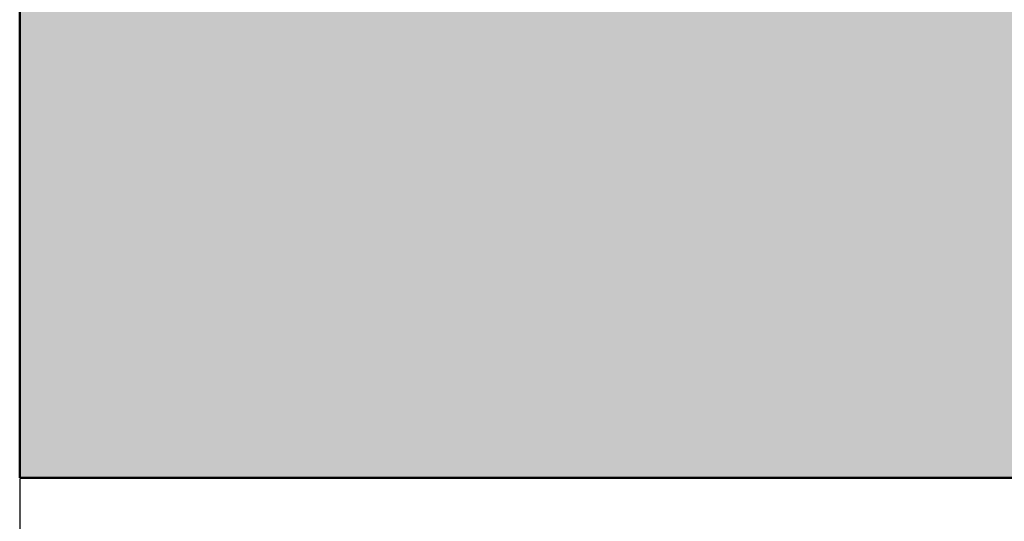
# Model space of a CAD drawing. Units: millimetres. Extents: x 0 to 2267, y 0 to 1823.
# Tile 12 of 256: x 1506 to 1590, y 1074 to 1116. Entities that reach past the tile are written whole.
import ezdxf

# ---------------------------------------------------------------- set-up
doc = ezdxf.new("R2010")
doc.units = ezdxf.units.MM
doc.header["$MEASUREMENT"] = 0
for name, color, linetype, lineweight in [('M-DIMS', 2, 'Continuous', 25), ('M-HATC', 252, 'Continuous', 18), ('M-OUTL', 7, 'Continuous', 50)]:
    doc.layers.add(name, color=color, linetype=linetype, lineweight=lineweight)
doc.styles.get("Standard").update_dxf_attribs({"font": 'arial.ttf'})
doc.dimstyles.get("Standard").update_dxf_attribs({"dimtxt": 7, "dimasz": 4, "dimexe": 0.18, "dimexo": 0.0625, "dimgap": 0.09, "dimtad": 0, "dimdec": 0, "dimzin": 0, "dimdsep": 46, "dimtxsty": 'Standard', "dimcen": 0.09, "dimadec": 0, "dimazin": 0, "dimtfac": 1, "dimtdec": 0, "dimtofl": 0, "dimtmove": 0, "dimatfit": 3, "dimfxl": 1, "dimtolj": 1, "dimtzin": 0, "dimarcsym": 0})

# ---------------------------------------------------------------- blocks, each defined once
blk = doc.blocks.new('*D2')
at = {"layer": 'Defpoints', "color": 0, "transparency": 16777216}
for p in [(1505.929, 1077.417), (1930.929, 1077.417), (1930.929, 906.787)]:
    blk.add_point(p, dxfattribs=at)
at = {"layer": 'M-DIMS', "color": 0, "lineweight": -2, "transparency": 16777216}
for p, q in [((1505.929, 1077.355), (1505.929, 906.607)), ((1930.929, 1077.355), (1930.929, 906.607)), ((1509.929, 906.787), (1710.439, 906.787)), ((1926.929, 906.787), (1726.419, 906.787))]:
    blk.add_line(p, q, dxfattribs=at)
at = {"layer": 'M-DIMS', "color": 0, "transparency": 16777216}
for points in [[(1509.929, 907.453), (1509.929, 906.12), (1505.929, 906.787)], [(1926.929, 907.453), (1926.929, 906.12), (1930.929, 906.787)]]:
    blk.add_solid(points, dxfattribs=at)
at = {"layer": 'M-DIMS', "color": 0, "transparency": 16777216, "insert": (1718.429, 906.787), "char_height": 7, "attachment_point": 5}
blk.add_mtext('\\A1;425', dxfattribs=at)

msp = doc.modelspace()

# ---------------------------------------------------------------- hatches: boundary and pattern name
at = {"layer": 'M-HATC'}
h = msp.add_hatch(color=256, dxfattribs=at)
h.dxf.hatch_style = 1
h.paths.add_polyline_path([(2065.771, 1618.062, 0.236068), (2055.771, 1638.062), (1381.087, 1638.062, 0.236068), (1371.087, 1618.062), (1371.087, 1603.062), (2055.771, 1603.062), (2065.771, 1603.062)])
h.paths.add_polyline_path([(2062.772, 1550.296), (2062.772, 1560.296), (1374.086, 1560.296), (1374.086, 1550.296), (1374.086, 1540.296), (1384.086, 1540.296), (1389.086, 1540.296), (2062.772, 1540.296)])
h.paths.add_polyline_path([(1930.929, 1282.766), (1505.929, 1282.766), (1587.628, 1235.597, 0.131652), (1600.128, 1232.247), (1836.73, 1232.247, 0.131652), (1849.23, 1235.597)])
h.paths.add_polyline_path([(1930.929, 1117.417), (1905.929, 1117.417), (1505.929, 1117.417), (1505.929, 1077.417), (1930.929, 1077.417)])

# ---------------------------------------------------------------- linework, layer by layer
at = {"layer": 'M-OUTL'}
for p, q in [((1505.929, 1117.417), (1505.929, 1077.417)), ((1505.929, 1077.417), (1930.929, 1077.417))]:
    msp.add_line(p, q, dxfattribs=at)

# ---------------------------------------------------------------- dimensions: what is measured, and where the dimension line sits
at = {"layer": 'M-DIMS'}
dim = msp.add_linear_dim(base=(1930.929, 906.787), p1=(1505.929, 1077.417), p2=(1930.929, 1077.417), dimstyle='Standard', override={"dimclrd": 0, "dimclre": 0, "dimclrt": 0}, dxfattribs=at)
dim.commit()
dim.dimension.update_dxf_attribs({"geometry": '*D2', "text_midpoint": (1718.429, 906.787)})

doc.saveas('drawing.dxf')
